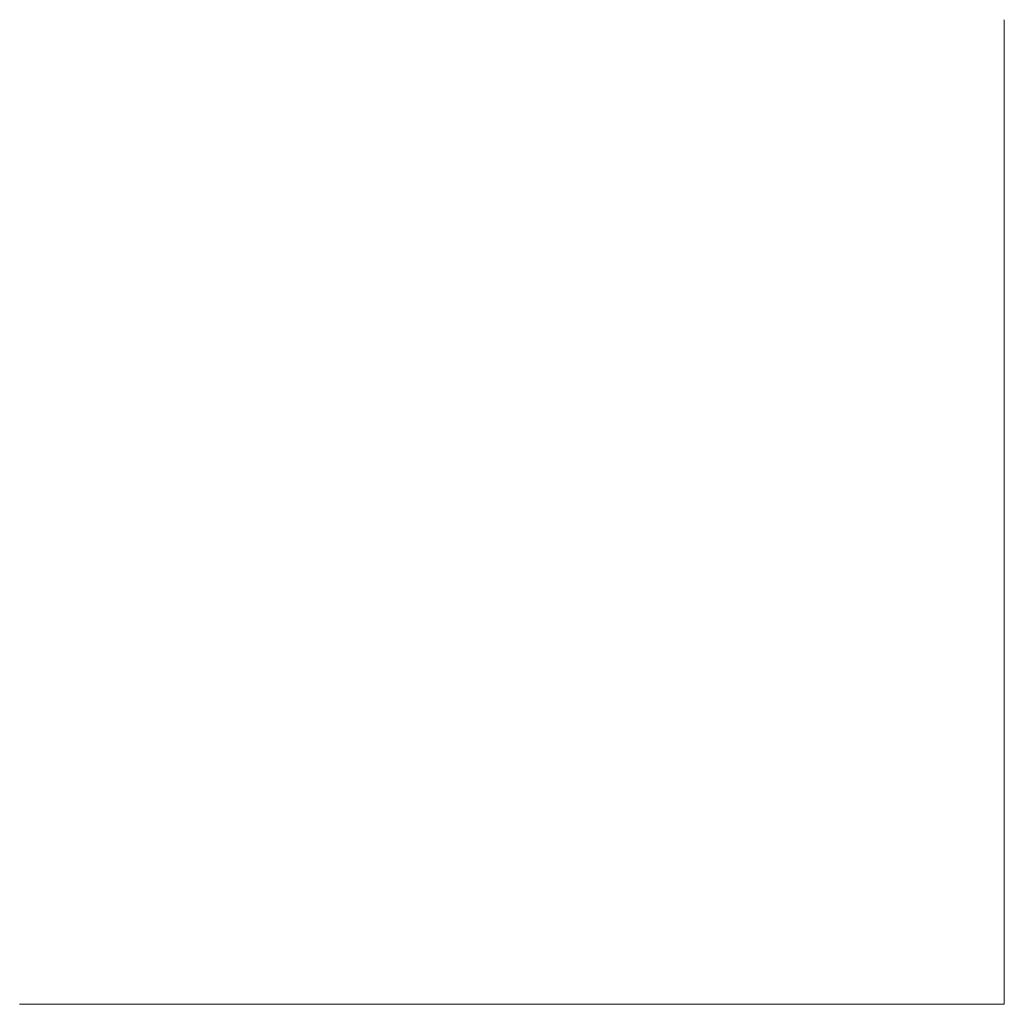
# Model space of a CAD drawing. Units: millimetres. Extents: x 482.6 to 494.6, y 784.6 to 796.6.
import ezdxf

# ---------------------------------------------------------------- set-up
doc = ezdxf.new("R2010")
doc.units = ezdxf.units.MM
doc.layers.add('M-CONS', color=8, linetype='Continuous', lineweight=13)

msp = doc.modelspace()

# ---------------------------------------------------------------- linework, layer by layer
at = {"layer": 'M-CONS'}
for p, q in [((494.612, 796.569, 12), (494.612, 784.569, 12)), ((494.612, 784.569, 12), (482.612, 784.569, 12))]:
    msp.add_line(p, q, dxfattribs=at)

doc.saveas('drawing.dxf')
